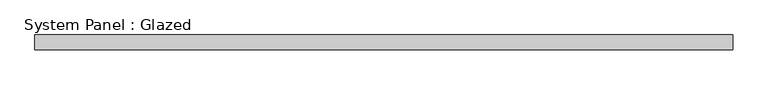
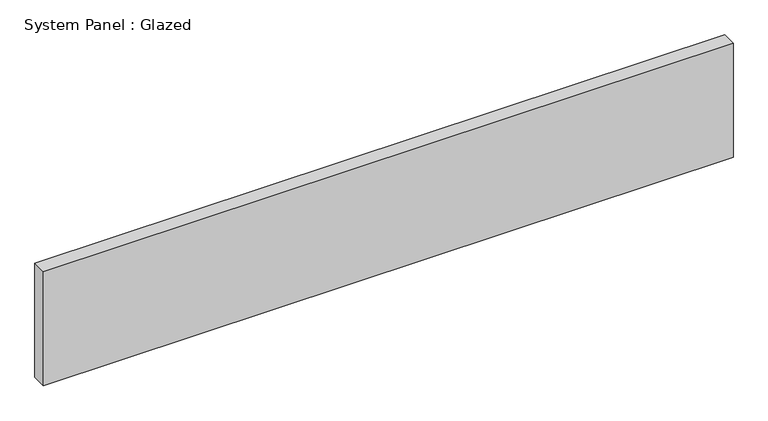
"""IFC4 building model written with IfcOpenShell, lengths in millimetres: plate geometry, System Panel : Glazed."""

from ifc_helpers import new_model, si_unit, origin, origin_with_axes, place, context, project, spatial, polyline, outline, extrude, source, transform, mapped, element, save


def system_panel_glazed_4e629a68(model_context):
    return source(origin(), model_context, "Body", "SweptSolid", [
        extrude(outline(polyline([(600.0750001, 19.05), (-600.0750001, 19.05), (-600.0750001, 44.45), (600.0750001, 44.45), (600.0750001, 19.05)])), origin_with_axes(), (0.0, 0.0, 1.0), 209.55),
    ])


if __name__ == "__main__":
    model = new_model("IFC4")
    model_context = context("Model", 3, world=origin())
    ifc_project = project(units=[si_unit("LENGTHUNIT", "METRE", prefix="MILLI")], contexts=[model_context])
    site = spatial("IfcSite", under=ifc_project)
    building = spatial("IfcBuilding", under=site)
    placement = place(None, origin())
    system_panel_glazed_shape = system_panel_glazed_4e629a68(model_context)
    element("IfcPlate", 1, ObjectType="System Panel : Glazed", at=placement, inside=building, context=model_context, shape_type="MappedRepresentation", body=[
        mapped(system_panel_glazed_shape, transform((0.0, 0.0, 0.0), x_axis=(1.0, 0.0, 0.0), y_axis=(0.0, 1.0, 0.0), z_axis=(0.0, 0.0, 1.0))),
    ])
    save(model, "model.ifc")

# Revit data of these elements
# Type "System Panel : Glazed"
#   Construction Type Id = "GSP4R"
#   Analytic Construction = "1/8 in Pilkington single glazing"
#   Visual Light Transmittance = 0.9
#   Solar Heat Gain Coefficient = 0.86
#   Heat Transfer Coefficient (U) = 1.18115 BTU/(h·ft²·°F)
#   Define Thermal Properties by = 1
# Element 1 (IfcPlate, "System Panel : Glazed")
#   Materials on its faces: "Glass"
# Materials
#   "Glass": class "Glass", colour RGB 0 128 192, transparency 0.75, Description = "Soda Lime Glass", Cost = 0
